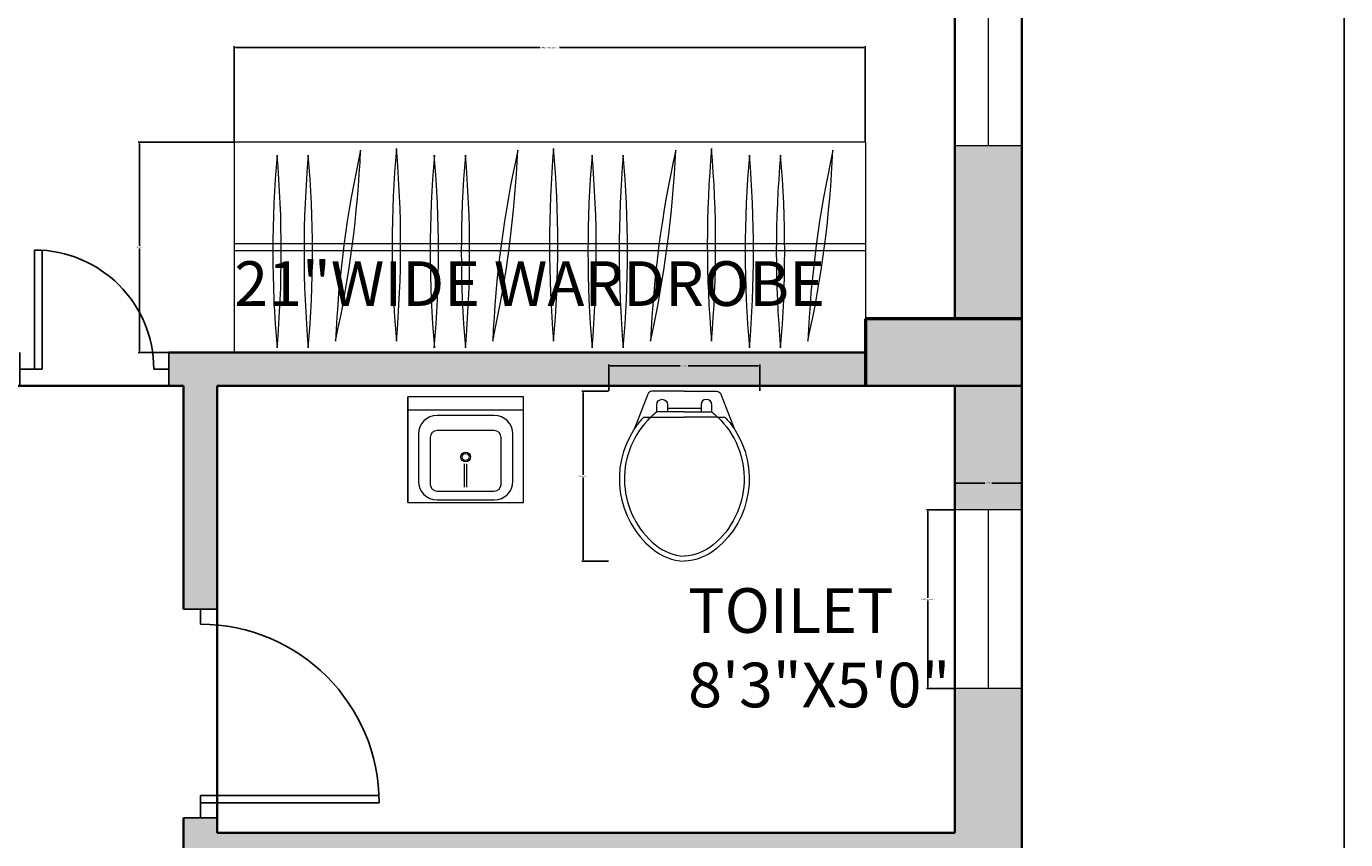
# Model space of a CAD drawing. Units: inches. Extents: x -28 to 485, y -861 to 54.
# Tile 13 of 14: x 308 to 485, y -208 to -99. Entities that reach past the tile are written whole.
import ezdxf

# ---------------------------------------------------------------- set-up
doc = ezdxf.new("R2010")
doc.units = ezdxf.units.IN
doc.header["$MEASUREMENT"] = 0
for name, color, linetype, lineweight in [('A-ANNO-DIMS', 2, 'Continuous', 18), ('A-ANNO-TEXT', 7, 'Continuous', 18), ('A-AREA-IDEN', 7, 'Continuous', 18), ('A-COLS', 7, 'Continuous', 50), ('A-COLS-PATT', 8, 'Continuous', 13), ('A-DOOR', 3, 'Continuous', 25), ('A-FLOR-CASE', 8, 'Continuous', 18), ('A-FLOR-FIXT', 9, 'Continuous', 18), ('A-GLAZ', 4, 'Continuous', 18), ('A-WALL', 7, 'Continuous', 35), ('A-WALL-PATT', 34, 'Continuous', 13)]:
    doc.layers.add(name, color=color, linetype=linetype, lineweight=lineweight)
doc.styles.get("Standard").update_dxf_attribs({"font": 'arial.ttf'})
doc.dimstyles.get("Standard").update_dxf_attribs({"dimtxt": 0.18, "dimasz": 0.18, "dimexe": 0.18, "dimexo": 0.0625, "dimgap": 0.09, "dimtad": 0, "dimtih": 1, "dimtoh": 1, "dimdec": 0, "dimzin": 0, "dimdsep": 46, "dimlunit": 3, "dimtxsty": 'Standard', "dimcen": 0.09, "dimadec": 0, "dimazin": 0, "dimtfac": 1, "dimtdec": 0, "dimtofl": 0, "dimtmove": 0, "dimatfit": 3, "dimfxl": 1, "dimtolj": 1, "dimtzin": 0, "dimarcsym": 0})

# ---------------------------------------------------------------- blocks, each defined once
blk = doc.blocks.new('М14 600х655')
for p, q in [((-655, 600), (-655, 0)), ((-655, 600), (-655, 0)), ((-655, 0), (-655, 600)), ((0, 600), (-655, 600)), ((0, 0), (0, 600)), ((0, 525), (-655, 525)), ((-165.1, 494.1), (-489.9, 494.1)), ((-595.8, 388.1), (-595.8, 121.3)), ((-165.4, 408.4), (-490.2, 408.4)), ((-59.2, 121.3), (-59.2, 388.1)), ((-528.4, 370.1), (-528.4, 103.3)), ((-127.2, 103.3), (-127.2, 370.1)), ((-333.5, 87.1), (-333.5, 219.6)), ((-321.5, 87.1), (-321.5, 219.6)), ((-655, 0), (-655, 0)), ((-655, 0), (-655, 0)), ((-655, 0), (0, 0)), ((-655, 0), (0, 0)), ((-490.2, 65.1), (-165.4, 65.1)), ((-489.9, 15.4), (-165.1, 15.4))]:
    blk.add_line(p, q)
for radius in [27.6, 19.3]:
    blk.add_circle((-327.5, 258.9), radius)
for centre, radius, start, end in [((-489.9, 388.1), 105.9, 90, 180), ((-165.1, 388.1), 105.9, 0, 90), ((-490.2, 370.1), 38.2, 90, 180), ((-165.4, 370.1), 38.2, 0, 90), ((-489.9, 121.3), 105.9, 180, 270), ((-490.2, 103.3), 38.2, 180, 270), ((-165.4, 103.3), 38.2, 270, 0), ((-165.1, 121.3), 105.9, 270, 0)]:
    blk.add_arc(centre, radius, start, end)
blk = doc.blocks.new('WARDROBE-HANGING')
for p, q in [((84.7, 28.23), (0, 28.23)), ((0, 28.23), (0, 0)), ((84.7, 28.23), (84.7, 0)), ((84.7, 14.59), (0, 14.59)), ((84.7, 13.65), (0, 13.65)), ((84.7, 0), (0, 0))]:
    blk.add_line(p, q)
for centre, start, end in [((-131.46, 33.65), 347.508, 357.5023), ((162.01, -4.96), 167.508, 177.5023), ((169.76, 14.46), 175.0028, 184.9972), ((-126.23, 14.46), 355.0028, 4.9972), ((-110.36, 33.65), 347.508, 357.5023), ((183.11, -4.96), 167.508, 177.5023), ((190.86, 14.46), 175.0028, 184.9972), ((-105.13, 14.46), 355.0028, 4.9972), ((204.29, -4.96), 167.508, 177.5023), ((-89.17, 33.65), 347.508, 357.5023), ((212.05, 14.46), 175.0028, 184.9972), ((-83.95, 14.46), 355.0028, 4.9972), ((225.4, -4.96), 167.508, 177.5023), ((-68.07, 33.65), 347.508, 357.5023), ((153.74, 13.55), 175.0028, 184.9972), ((-142.25, 13.55), 355.0028, 4.9972), ((157.93, 13.55), 175.0028, 184.9972), ((-138.07, 13.55), 355.0028, 4.9972), ((174.85, 13.55), 175.0028, 184.9972), ((-121.15, 13.55), 355.0028, 4.9972), ((179.03, 13.55), 175.0028, 184.9972), ((-116.97, 13.55), 355.0028, 4.9972), ((196.03, 13.55), 175.0028, 184.9972), ((-99.97, 13.55), 355.0028, 4.9972), ((200.21, 13.55), 175.0028, 184.9972), ((-95.78, 13.55), 355.0028, 4.9972), ((217.13, 13.55), 175.0028, 184.9972), ((-78.86, 13.55), 355.0028, 4.9972), ((221.31, 13.55), 175.0028, 184.9972), ((-74.68, 13.55), 355.0028, 4.9972)]:
    blk.add_arc(centre, 148.56, start, end)
blk = doc.blocks.new('WC-FLOOR-MOUNTED')
for p, q in [((3.27, 19.35), (4.23, 19.35)), ((4.23, 19.35), (8.71, 19.35)), ((13.2, 19.35), (8.71, 19.35)), ((13.2, 19.35), (14.16, 19.35))]:
    blk.add_line(p, q)
for points in [[(8.71, 22.81), (4.36, 22.81, 0.31031), (3.82, 22.44), (2.03, 17.79, 0.209071)], [(5.01, 20.04), (5.01, 21, -1), (6.47, 21), (6.47, 20.5)], [(8.71, 22.81), (13.07, 22.81, -0.31031), (13.6, 22.44), (15.39, 17.79, -0.209071)], [(12.41, 20.04), (12.41, 21, 1), (10.96, 21), (10.96, 20.5)], [(5.01, 20.04, 0.022712), (4.23, 19.35, 0.162618)], [(8.71, 20.04), (5.01, 20.04, 0.022712)], [(8.71, 20.04), (12.41, 20.04, -0.476108)], [(12.41, 20.04, -0.022712), (13.2, 19.35, -0.162618)], [(2.03, 17.79, 0.383919), (4.43, 1.64, 0.163732), (8.71, 0, 0.359733)], [(3.77, 18.89, 0.431639), (4.86, 2.17, 0.162618), (8.71, 0.68, 0.470877)], [(3.27, 19.35, 0.040937), (2.03, 17.79, 0.163732)], [(4.23, 19.35, 0.014165), (3.77, 18.89, 0.162618)], [(13.2, 19.35, -0.448546), (12.57, 2.17, -0.162618), (8.71, 0.68, -0.470877)], [(15.39, 17.79, -0.383919), (13, 1.64, -0.163732), (8.71, 0, -0.359733)], [(14.16, 19.35, -0.040937), (15.39, 17.79, -0.163732)]]:
    blk.add_lwpolyline(points, format="xyb")
for points in [[(10.96, 20.5), (6.47, 20.5)], [(6.47, 20.5), (6.47, 20.04)], [(10.96, 20.5), (10.96, 20.04)]]:
    blk.add_lwpolyline(points)
blk = doc.blocks.new('DOOR-SWING-NARROW')
for p, q in [((17, 2.25), (17, 18.25)), ((18, 2.25), (18, 18.25)), ((0, 2.25), (0, 4.5)), ((20, 4.5), (20, 0)), ((0, 2.25), (0, 0)), ((0, 2.25), (2, 2.25)), ((17, 2.25), (18, 2.25)), ((20, 2.25), (18, 2.25))]:
    blk.add_line(p, q)
blk.add_arc((18, 2.25), 16, 90, 180)
blk = doc.blocks.new('DOOR-SWING-24')
for p, q in [((2, 2.25), (2, 26.25)), ((3, 2.25), (3, 26.25)), ((0, 4.5), (0, 0)), ((28, 2.25), (28, 4.5)), ((0, 2.25), (2, 2.25)), ((2, 2.25), (3, 2.25)), ((26, 2.25), (28, 2.25)), ((28, 2.25), (28, 0))]:
    blk.add_line(p, q)
blk.add_arc((2, 2.25), 24, 0, 90)
blk = doc.blocks.new('WINDOW-60IN')
for p, q in [((0, 60), (0, 0)), ((9, 60), (0, 60)), ((4.5, 60), (4.5, 0)), ((9, 0), (9, 60)), ((0, 0), (9, 0))]:
    blk.add_line(p, q)
blk = doc.blocks.new('WINDOW-24IN')
for p, q in [((0, 24), (0, 0)), ((9, 24), (0, 24)), ((4.5, 24), (4.5, 0)), ((9, 0), (9, 24)), ((9, 0), (0, 0))]:
    blk.add_line(p, q)
blk = doc.blocks.new('*D26')
at = {"layer": 'A-ANNO-DIMS', "color": 0, "lineweight": -2, "transparency": 16777216}
for p, q in [((335.58, -114.57), (335.58, -101.75)), ((335.76, -101.93), (376.63, -101.93)), ((420.1, -101.93), (379.24, -101.93)), ((420.28, -114.57), (420.28, -101.75))]:
    blk.add_line(p, q, dxfattribs=at)
at = {"layer": 'A-ANNO-DIMS', "color": 0, "transparency": 16777216}
for points in [[(335.76, -101.9), (335.76, -101.96), (335.58, -101.93)], [(420.1, -101.9), (420.1, -101.96), (420.28, -101.93)]]:
    blk.add_solid(points, dxfattribs=at)
at = {"layer": 'Defpoints', "color": 0, "transparency": 16777216}
for p in [(420.28, -101.93), (335.58, -114.63), (420.28, -114.63)]:
    blk.add_point(p, dxfattribs=at)
at = {"layer": 'A-ANNO-DIMS', "color": 0, "transparency": 16777216, "insert": (377.93, -101.93), "char_height": 0.18, "attachment_point": 5}
blk.add_mtext('\\A1;WARDROBE 85 TYP.', dxfattribs=at)
blk = doc.blocks.new('*D27')
at = {"layer": 'A-ANNO-DIMS', "color": 0, "lineweight": -2, "transparency": 16777216}
for p, q in [((335.52, -114.63), (322.7, -114.63)), ((322.88, -114.81), (322.88, -128.57)), ((322.88, -142.69), (322.88, -128.93)), ((335.52, -142.87), (322.7, -142.87))]:
    blk.add_line(p, q, dxfattribs=at)
at = {"layer": 'A-ANNO-DIMS', "color": 0, "transparency": 16777216}
for points in [[(322.85, -114.81), (322.91, -114.81), (322.88, -114.63)], [(322.85, -142.69), (322.91, -142.69), (322.88, -142.87)]]:
    blk.add_solid(points, dxfattribs=at)
at = {"layer": 'Defpoints', "color": 0, "transparency": 16777216}
for p in [(322.88, -114.63), (335.58, -114.63), (335.58, -142.87)]:
    blk.add_point(p, dxfattribs=at)
at = {"layer": 'A-ANNO-DIMS', "color": 0, "transparency": 16777216, "insert": (322.88, -128.75), "char_height": 0.18, "attachment_point": 5}
blk.add_mtext('\\A1;28 TYP.', dxfattribs=at)
blk = doc.blocks.new('*D30')
at = {"layer": 'A-ANNO-DIMS', "color": 0, "lineweight": -2, "transparency": 16777216}
for p, q in [((385.79, -148.09), (382.25, -148.09)), ((382.43, -148.27), (382.43, -159.31)), ((382.43, -170.71), (382.43, -159.67)), ((385.79, -170.89), (382.25, -170.89))]:
    blk.add_line(p, q, dxfattribs=at)
at = {"layer": 'A-ANNO-DIMS', "color": 0, "transparency": 16777216}
for points in [[(382.4, -148.27), (382.46, -148.27), (382.43, -148.09)], [(382.4, -170.71), (382.46, -170.71), (382.43, -170.89)]]:
    blk.add_solid(points, dxfattribs=at)
at = {"layer": 'Defpoints', "color": 0, "transparency": 16777216}
for p in [(382.43, -148.09), (385.85, -148.09), (385.85, -170.89)]:
    blk.add_point(p, dxfattribs=at)
at = {"layer": 'A-ANNO-DIMS', "color": 0, "transparency": 16777216, "insert": (382.43, -159.49), "char_height": 0.18, "attachment_point": 5}
blk.add_mtext('\\A1;WC 23 TYP.', dxfattribs=at)
blk = doc.blocks.new('*D31')
at = {"layer": 'A-ANNO-DIMS', "color": 0, "lineweight": -2, "transparency": 16777216}
for p, q in [((385.85, -148.03), (385.85, -144.49)), ((386.03, -144.67), (395.45, -144.67)), ((405.93, -144.67), (396.51, -144.67)), ((406.11, -148.03), (406.11, -144.49))]:
    blk.add_line(p, q, dxfattribs=at)
at = {"layer": 'A-ANNO-DIMS', "color": 0, "transparency": 16777216}
for points in [[(386.03, -144.64), (386.03, -144.7), (385.85, -144.67)], [(405.93, -144.64), (405.93, -144.7), (406.11, -144.67)]]:
    blk.add_solid(points, dxfattribs=at)
at = {"layer": 'Defpoints', "color": 0, "transparency": 16777216}
for p in [(406.11, -144.67), (385.85, -148.09), (406.11, -148.09)]:
    blk.add_point(p, dxfattribs=at)
at = {"layer": 'A-ANNO-DIMS', "color": 0, "transparency": 16777216, "insert": (395.98, -144.67), "char_height": 0.18, "attachment_point": 5}
blk.add_mtext('\\A1;20 TYP.', dxfattribs=at)
blk = doc.blocks.new('*D34')
at = {"layer": 'A-ANNO-DIMS', "color": 0, "lineweight": -2, "transparency": 16777216}
for p, q in [((432.22, -164.01), (428.5, -164.01)), ((428.68, -164.19), (428.68, -175.82)), ((428.68, -187.83), (428.68, -176.19)), ((432.22, -188.01), (428.5, -188.01))]:
    blk.add_line(p, q, dxfattribs=at)
at = {"layer": 'A-ANNO-DIMS', "color": 0, "transparency": 16777216}
for points in [[(428.65, -164.19), (428.71, -164.19), (428.68, -164.01)], [(428.65, -187.83), (428.71, -187.83), (428.68, -188.01)]]:
    blk.add_solid(points, dxfattribs=at)
at = {"layer": 'Defpoints', "color": 0, "transparency": 16777216}
for p in [(428.68, -164.01), (432.28, -164.01), (432.28, -188.01)]:
    blk.add_point(p, dxfattribs=at)
at = {"layer": 'A-ANNO-DIMS', "color": 0, "transparency": 16777216, "insert": (428.68, -176.01), "char_height": 0.18, "attachment_point": 5}
blk.add_mtext('\\A1;WINDOW 24 TYP.', dxfattribs=at)
blk = doc.blocks.new('*D35')
at = {"layer": 'A-ANNO-DIMS', "color": 0, "lineweight": -2, "transparency": 16777216}
for p, q in [((432.28, -163.95), (432.28, -160.23)), ((432.46, -160.41), (436.33, -160.41)), ((441.1, -160.41), (437.24, -160.41)), ((441.28, -163.95), (441.28, -160.23))]:
    blk.add_line(p, q, dxfattribs=at)
at = {"layer": 'A-ANNO-DIMS', "color": 0, "transparency": 16777216}
for points in [[(432.46, -160.38), (432.46, -160.44), (432.28, -160.41)], [(441.1, -160.38), (441.1, -160.44), (441.28, -160.41)]]:
    blk.add_solid(points, dxfattribs=at)
at = {"layer": 'Defpoints', "color": 0, "transparency": 16777216}
for p in [(441.28, -160.41), (432.28, -164.01), (441.28, -164.01)]:
    blk.add_point(p, dxfattribs=at)
at = {"layer": 'A-ANNO-DIMS', "color": 0, "transparency": 16777216, "insert": (436.78, -160.41), "char_height": 0.18, "attachment_point": 5}
blk.add_mtext('\\A1;9 TYP.', dxfattribs=at)
blk = doc.blocks.new('*D53')
at = {"layer": 'A-ANNO-DIMS', "color": 0, "lineweight": -2, "transparency": 16777216}
for p, q in [((441.35, 10.13), (484.71, 10.13)), ((484.53, 9.95), (484.53, -403.68)), ((484.53, -817.69), (484.53, -404.05)), ((441.35, -817.87), (484.71, -817.87))]:
    blk.add_line(p, q, dxfattribs=at)
at = {"layer": 'A-ANNO-DIMS', "color": 0, "transparency": 16777216}
for points in [[(484.5, 9.95), (484.56, 9.95), (484.53, 10.13)], [(484.5, -817.69), (484.56, -817.69), (484.53, -817.87)]]:
    blk.add_solid(points, dxfattribs=at)
at = {"layer": 'Defpoints', "color": 0, "transparency": 16777216}
for p in [(441.28, 10.13), (441.28, -817.87), (484.53, -817.87)]:
    blk.add_point(p, dxfattribs=at)
at = {"layer": 'A-ANNO-DIMS', "color": 0, "transparency": 16777216, "insert": (484.53, -403.87), "char_height": 0.18, "attachment_point": 5}
blk.add_mtext('\\A1;828', dxfattribs=at)

msp = doc.modelspace()

# ---------------------------------------------------------------- hatches: boundary and pattern name
at = {"layer": 'A-COLS-PATT'}
h = msp.add_hatch(color=256, dxfattribs=at)
h.dxf.hatch_style = 1
h.paths.add_polyline_path([(36.285, 10.133), (15.285, 10.133), (15.285, 1.133), (36.285, 1.133)])
h.paths.add_polyline_path([(160.785, 10.133), (139.785, 10.133), (139.785, 1.133), (160.785, 1.133)])
h.paths.add_polyline_path([(316.785, 10.133), (295.785, 10.133), (295.785, 1.133), (316.785, 1.133)])
h.paths.add_polyline_path([(441.285, 10.133), (420.285, 10.133), (420.285, 1.133), (441.285, 1.133)])
h.paths.add_polyline_path([(441.285, -138.367), (432.285, -138.367), (420.285, -138.367), (420.285, -147.367), (441.285, -147.367)])
h.paths.add_polyline_path([(304.785, -130.867), (295.785, -130.867), (295.785, -147.367), (304.785, -147.367), (304.785, -142.867)])
h.paths.add_polyline_path([(160.785, -130.867), (151.785, -130.867), (151.785, -142.867), (151.785, -147.367), (160.785, -147.367)])
h.paths.add_polyline_path([(36.285, -138.367), (24.285, -138.367), (15.285, -138.367), (15.285, -147.367), (36.285, -147.367)])
h.paths.add_polyline_path([(36.285, -355.867), (15.285, -355.867), (15.285, -364.867), (36.285, -364.867)])
h.paths.add_polyline_path([(160.785, -355.867), (139.785, -355.867), (139.785, -364.867), (160.785, -364.867)])
h.paths.add_polyline_path([(316.785, -355.867), (300.285, -355.867), (295.785, -355.867), (295.785, -364.867), (316.785, -364.867)])
at = {"layer": 'A-WALL-PATT'}
h = msp.add_hatch(color=256, dxfattribs=at)
h.dxf.hatch_style = 1
h.paths.add_polyline_path([(160.785, -808.867), (160.785, -817.867), (295.785, -817.867), (295.785, -808.867)])
h.paths.add_polyline_path([(316.785, -817.867), (323.776, -817.867), (323.776, -808.867), (316.785, -808.867)])
h.paths.add_polyline_path([(420.285, -817.867), (420.285, -808.867), (383.776, -808.867), (383.776, -817.867)])
h.paths.add_polyline_path([(432.285, -808.867), (441.285, -808.867), (441.285, -702.966), (432.285, -702.966), (432.285, -708.367), (397.785, -708.367), (397.785, -710.617), (397.785, -712.867), (432.285, -712.867)])
h.paths.add_polyline_path([(300.285, -712.867), (329.285, -712.867), (329.285, -710.617), (329.285, -708.367), (295.785, -708.367), (295.785, -808.867), (300.285, -808.867)])
h.paths.add_polyline_path([(160.785, -698.867), (158.535, -698.867), (156.285, -698.867), (156.285, -808.867), (160.785, -808.867)])
h.paths.add_polyline_path([(36.285, -808.867), (36.285, -817.867), (79.721, -817.867), (79.721, -808.867)])
h.paths.add_polyline_path([(15.285, -808.867), (24.285, -808.867), (24.285, -739.09), (15.285, -739.09)])
h.paths.add_polyline_path([(24.285, -640.781), (15.285, -640.781), (15.285, -679.09), (24.285, -679.09), (24.285, -664.867), (89.285, -664.867), (89.285, -662.617), (89.285, -660.367), (24.285, -660.367)])
h.paths.add_polyline_path([(15.285, -616.781), (24.285, -616.781), (24.285, -600.367), (15.285, -600.367)])
h.paths.add_polyline_path([(36.285, -595.867), (36.285, -600.367), (123.285, -600.367), (123.285, -660.367), (117.285, -660.367), (117.285, -664.867), (156.285, -664.867), (156.285, -670.867), (160.785, -670.867), (160.785, -660.367), (127.785, -660.367), (127.785, -600.367), (129.785, -600.367), (129.785, -598.117), (129.785, -595.867)])
h.paths.add_polyline_path([(367.785, -664.867), (363.285, -664.867), (363.285, -708.367), (357.285, -708.367), (357.285, -712.867), (369.785, -712.867), (369.785, -708.367), (367.785, -708.367)])
h.paths.add_polyline_path([(432.285, -664.867), (432.285, -666.966), (441.285, -666.966), (441.285, -642.367), (432.285, -642.367), (432.285, -660.367), (328.785, -660.367), (328.785, -664.867), (363.285, -664.867)])
h.paths.add_polyline_path([(333.285, -600.367), (420.285, -600.367), (420.285, -595.867), (326.785, -595.867), (326.785, -600.367), (328.785, -600.367), (328.785, -630.367), (331.035, -630.367), (333.285, -630.367)])
h.paths.add_polyline_path([(441.285, -600.367), (432.285, -600.367), (432.285, -618.367), (441.285, -618.367)])
h.paths.add_polyline_path([(432.285, -591.367), (441.285, -591.367), (441.285, -547.793), (432.285, -547.793)])
h.paths.add_polyline_path([(295.785, -588.367), (300.238, -588.367), (300.285, -583.867), (300.285, -451.867), (295.785, -451.867)])
h.paths.add_polyline_path([(420.285, -451.867), (420.285, -442.867), (316.785, -442.867), (316.785, -451.867)])
h.paths.add_polyline_path([(432.285, -487.793), (441.285, -487.793), (441.285, -451.867), (432.285, -451.867)])
h.paths.add_polyline_path([(432.285, -442.867), (441.285, -442.867), (441.285, -364.867), (432.285, -364.867)])
h.paths.add_polyline_path([(261.785, -451.867), (261.785, -447.367), (261.785, -444.758), (261.785, -442.867), (160.785, -442.867), (160.785, -451.867)])
h.paths.add_polyline_path([(139.785, -451.867), (139.785, -442.867), (36.285, -442.867), (36.285, -451.867)])
h.paths.add_polyline_path([(15.285, -491.617), (24.285, -491.617), (24.285, -451.867), (15.285, -451.867)])
h.paths.add_polyline_path([(24.285, -551.617), (15.285, -551.617), (15.285, -591.367), (24.285, -591.367)])
h.paths.add_polyline_path([(160.785, -451.867), (156.285, -451.867), (156.285, -588.367), (160.785, -588.367)])
h.paths.add_polyline_path([(139.785, -364.867), (139.785, -355.867), (36.285, -355.867), (36.285, -364.867)])
h.paths.add_polyline_path([(24.285, -364.867), (15.285, -364.867), (15.285, -373.867), (24.285, -373.867)])
h.paths.add_polyline_path([(15.285, -433.867), (15.285, -442.867), (24.285, -442.867), (24.285, -433.867)])
h.paths.add_polyline_path([(261.785, -364.867), (261.785, -360.367), (261.785, -355.867), (160.785, -355.867), (160.785, -364.867)])
h.paths.add_polyline_path([(295.785, -355.867), (289.785, -355.867), (289.785, -364.867), (295.785, -364.867)])
h.paths.add_polyline_path([(295.785, -355.867), (300.285, -355.867), (300.285, -259.867), (333.285, -259.867), (333.285, -257.617), (333.285, -255.367), (300.285, -255.367), (300.285, -207.367), (295.785, -207.367)])
h.paths.add_polyline_path([(420.285, -364.867), (420.285, -355.867), (316.785, -355.867), (316.785, -364.867)])
h.paths.add_polyline_path([(24.285, -311.192), (15.285, -311.192), (15.285, -355.867), (24.285, -355.867)])
h.paths.add_polyline_path([(24.285, -211.867), (54.144, -211.867), (54.144, -207.367), (24.285, -207.367), (24.285, -187.772), (15.285, -187.772), (15.285, -251.192), (24.285, -251.192)])
h.paths.add_polyline_path([(82.144, -207.367), (82.144, -209.617), (82.144, -211.867), (127.785, -211.867), (127.785, -147.367), (129.785, -147.367), (129.785, -145.117), (129.785, -142.867), (36.285, -142.867), (36.285, -147.367), (123.285, -147.367), (123.285, -207.367)])
h.paths.add_polyline_path([(160.785, -207.367), (156.285, -207.367), (156.285, -355.867), (160.785, -355.867)])
h.paths.add_polyline_path([(24.285, 1.133), (15.285, 1.133), (15.285, -54.408), (24.285, -54.408)])
h.paths.add_polyline_path([(36.285, 10.133), (36.285, 1.133), (70.235, 1.133), (70.235, 10.133)])
h.paths.add_polyline_path([(15.285, -138.367), (24.285, -138.367), (24.285, -114.408), (15.285, -114.408)])
h.paths.add_polyline_path([(24.285, -147.367), (15.285, -147.367), (15.285, -163.772), (24.285, -163.772)])
h.paths.add_polyline_path([(156.285, -130.867), (160.785, -130.867), (160.785, 1.133), (156.285, 1.133)])
h.paths.add_polyline_path([(130.235, 1.133), (139.785, 1.133), (139.785, 10.133), (130.235, 10.133)])
h.paths.add_polyline_path([(316.785, 10.133), (316.785, 1.133), (328.097, 1.133), (328.097, 10.133)])
h.paths.add_polyline_path([(300.285, 1.133), (295.785, 1.133), (295.785, -130.867), (300.285, -130.867)])
h.paths.add_polyline_path([(420.285, -147.367), (420.285, -142.867), (326.785, -142.867), (326.785, -145.117), (326.785, -147.367), (328.785, -147.367), (328.785, -177.367), (331.035, -177.367), (333.285, -177.367), (333.285, -147.367)])
h.paths.add_polyline_path([(333.285, -207.367), (333.285, -205.367), (328.785, -205.367), (328.785, -211.867), (363.285, -211.867), (363.285, -255.367), (361.285, -255.367), (361.285, -259.867), (369.785, -259.867), (369.785, -255.367), (367.785, -255.367), (367.785, -211.867), (432.285, -211.867), (432.285, -214.893), (441.285, -214.893), (441.285, -188.008), (432.285, -188.008), (432.285, -207.367)])
h.paths.add_polyline_path([(441.285, -250.893), (432.285, -250.893), (432.285, -255.367), (397.785, -255.367), (397.785, -257.617), (397.785, -259.867), (432.285, -259.867), (432.285, -355.867), (441.285, -355.867)])
h.paths.add_polyline_path([(432.285, -138.367), (441.285, -138.367), (441.285, -115.099), (432.285, -115.099)])
h.paths.add_polyline_path([(441.285, -147.367), (432.285, -147.367), (432.285, -164.008), (441.285, -164.008)])
h.paths.add_polyline_path([(420.285, 1.133), (420.285, 10.133), (388.097, 10.133), (388.097, 1.133)])
h.paths.add_polyline_path([(432.285, -55.099), (441.285, -55.099), (441.285, 1.133), (432.285, 1.133)])

# ---------------------------------------------------------------- linework, layer by layer
at = {"layer": 'A-COLS'}
for p, q in [((432.285, -138.367), (420.285, -138.367)), ((420.285, -138.367), (420.285, -147.367)), ((441.285, -138.367), (432.285, -138.367))]:
    msp.add_line(p, q, dxfattribs=at)
at = {"layer": 'A-DOOR'}
msp.add_line((328.785, -145.117), (328.785, -145.117), dxfattribs=at)
at = {"layer": 'A-WALL'}
for p, q in [((441.285, 10.133), (441.285, -817.867)), ((432.285, 1.133), (432.285, -138.367)), ((326.785, -142.867), (420.285, -142.867)), ((295.785, -147.367), (328.785, -147.367)), ((328.785, -147.367), (328.785, -177.367)), ((333.285, -147.367), (333.285, -207.367)), ((333.285, -147.367), (441.285, -147.367)), ((432.285, -147.367), (432.285, -207.367)), ((328.785, -205.367), (328.785, -211.867)), ((333.285, -207.367), (432.285, -207.367))]:
    msp.add_line(p, q, dxfattribs=at)

# ---------------------------------------------------------------- block references
at = {"layer": 'A-DOOR', "extrusion": (0, 0, -1), "zscale": -1}
msp.add_blockref('DOOR-SWING-NARROW', (-326.784, -147.367), dxfattribs=at)
at = {"layer": 'A-DOOR', "extrusion": (0, 0, -1), "zscale": -1, "rotation": 90}
msp.add_blockref('DOOR-SWING-24', (-328.785, -205.367), dxfattribs=at)
at = {"layer": 'A-FLOR-CASE'}
msp.add_blockref('WARDROBE-HANGING', (335.582, -142.867), dxfattribs=at)
at = {"layer": 'A-FLOR-FIXT'}
msp.add_blockref('WC-FLOOR-MOUNTED', (387.267, -170.895), dxfattribs=at)
at = {"layer": 'A-FLOR-FIXT', "xscale": 0.0236562783211592, "yscale": 0.0236562783211592, "zscale": 0.0236562783211592}
msp.add_blockref('М14 600х655', (374.393, -163.028), dxfattribs=at)
at = {"layer": 'A-GLAZ'}
for name, p in [('WINDOW-60IN', (432.285, -115.099)), ('WINDOW-24IN', (432.285, -188.008))]:
    msp.add_blockref(name, p, dxfattribs=at)

# ---------------------------------------------------------------- texts
at = {"layer": 'A-ANNO-TEXT', "insert": (335.581, -130.628), "char_height": 6, "attachment_point": 1}
msp.add_mtext('21"WIDE WARDROBE', dxfattribs=at)
at = {"layer": 'A-AREA-IDEN', "insert": (396.506, -174.529), "char_height": 6, "attachment_point": 1}
msp.add_mtext('TOILET\\P8\'3"X5\'0"', dxfattribs=at)

# ---------------------------------------------------------------- dimensions: what is measured, and where the dimension line sits
at = {"layer": 'A-ANNO-DIMS'}
dim = msp.add_linear_dim(base=(484.535, -817.867), p1=(441.285, 10.133), p2=(441.285, -817.867), angle=90, dimstyle='Standard', override={"dimdec": 0, "dimlfac": 1, "dimrnd": 0, "dimzin": 0, "dimdsep": 46, "dimlunit": 2}, dxfattribs=at)
dim.commit()
dim.dimension.update_dxf_attribs({"geometry": '*D53', "text_midpoint": (484.535, -403.867)})
for base, p1, p2, text, picture, middle in [((420.285, -101.927), (335.581, -114.633), (420.285, -114.633), 'WARDROBE <> TYP.', '*D26', (377.933, -101.927)), ((406.111, -144.667), (385.849, -148.088), (406.111, -148.088), '<> TYP.', '*D31', (395.98, -144.667)), ((441.285, -160.408), (432.285, -164.008), (441.285, -164.008), '<> TYP.', '*D35', (436.785, -160.408))]:
    dim = msp.add_linear_dim(base=base, p1=p1, p2=p2, text=text, dimstyle='Standard', override={"dimdec": 0, "dimlfac": 1, "dimrnd": 0, "dimzin": 0, "dimdsep": 46, "dimlunit": 2}, dxfattribs=at)
    dim.commit()
    dim.dimension.update_dxf_attribs({"geometry": picture, "text_midpoint": middle})
for base, p1, p2, text, picture, middle in [((322.876, -114.633), (335.581, -142.867), (335.581, -114.633), '<> TYP.', '*D27', (322.876, -128.75)), ((382.428, -148.088), (385.849, -170.895), (385.849, -148.088), 'WC <> TYP.', '*D30', (382.428, -159.491)), ((428.685, -164.008), (432.285, -188.008), (432.285, -164.008), 'WINDOW <> TYP.', '*D34', (428.685, -176.008))]:
    dim = msp.add_linear_dim(base=base, p1=p1, p2=p2, angle=90, text=text, dimstyle='Standard', override={"dimdec": 0, "dimlfac": 1, "dimrnd": 0, "dimzin": 0, "dimdsep": 46, "dimlunit": 2}, dxfattribs=at)
    dim.commit()
    dim.dimension.update_dxf_attribs({"geometry": picture, "text_midpoint": middle})

doc.saveas('drawing.dxf')
